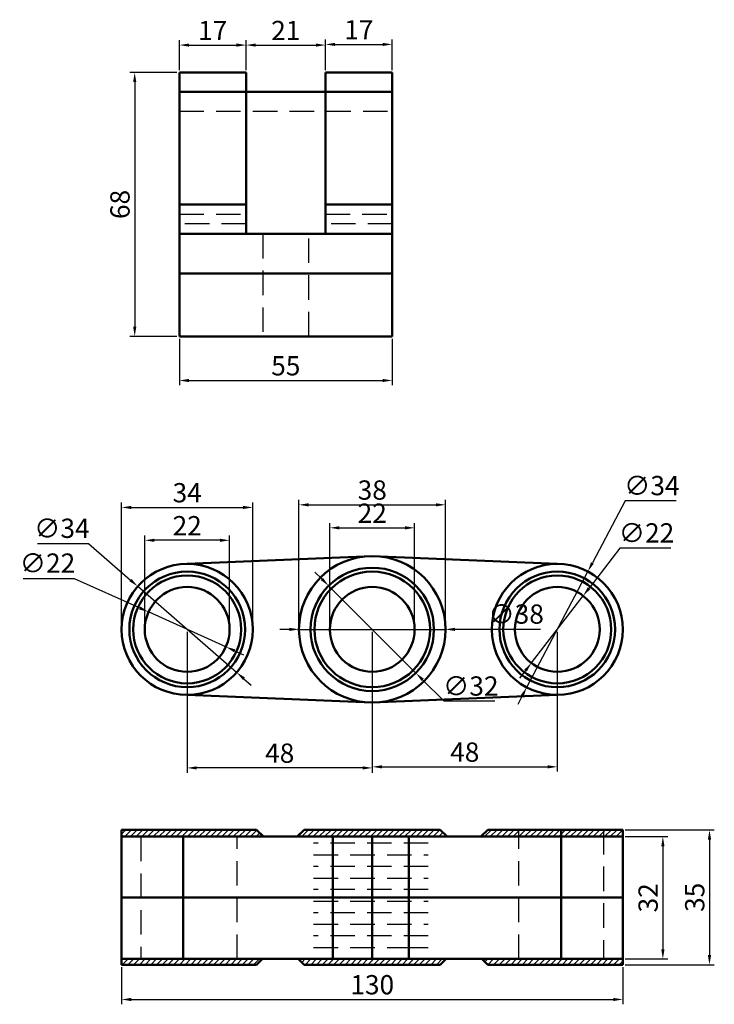
# Model space of a CAD drawing. Units: millimetres. Extents: x 1338 to 1892, y 1867 to 2306.
# Tile 3 of 3: x 1712 to 1892, y 2050 to 2306. Entities that reach past the tile are written whole.
import ezdxf

# ---------------------------------------------------------------- set-up
doc = ezdxf.new("R2010")
doc.units = ezdxf.units.MM
doc.linetypes.add('HIDDEN', pattern=[9.525, 6.35, -3.175])
for name, color, linetype, lineweight in [('M-DIMS', 2, 'Continuous', 25), ('M-HATC', 8, 'Continuous', 18), ('M-HIDN', 4, 'HIDDEN', 25), ('M-OUTL', 7, 'Continuous', 50)]:
    doc.layers.add(name, color=color, linetype=linetype, lineweight=lineweight)
doc.styles.get("Standard").update_dxf_attribs({"font": 'arial.ttf'})
doc.dimstyles.new('ISO-25', dxfattribs={"dimtxt": 5, "dimasz": 2.5, "dimexe": 1.25, "dimexo": 0.625, "dimtad": 1, "dimtoh": 1, "dimdec": 0, "dimtxsty": 'Standard', "dimcen": 2.5, "dimadec": 0, "dimazin": 0, "dimtfac": 1, "dimtdec": 0, "dimtmove": 0, "dimatfit": 3, "dimfxl": 1, "dimarcsym": 0})

# ---------------------------------------------------------------- blocks, each defined once
blk = doc.blocks.new('*D26')
at = {"layer": 'Defpoints', "color": 0, "transparency": 16777216}
for p in [(1771.04, 2299.06), (1753.74, 2291.96), (1771.04, 2291.96)]:
    blk.add_point(p, dxfattribs=at)
at = {"layer": 'M-DIMS', "color": 0, "lineweight": -2, "transparency": 16777216}
for p, q in [((1753.74, 2292.59), (1753.74, 2300.31)), ((1756.24, 2299.06), (1768.54, 2299.06)), ((1771.04, 2292.59), (1771.04, 2300.31))]:
    blk.add_line(p, q, dxfattribs=at)
at = {"layer": 'M-DIMS', "color": 0, "transparency": 16777216}
for points in [[(1756.24, 2299.48), (1756.24, 2298.65), (1753.74, 2299.06)], [(1768.54, 2299.48), (1768.54, 2298.65), (1771.04, 2299.06)]]:
    blk.add_solid(points, dxfattribs=at)
at = {"layer": 'M-DIMS', "color": 0, "transparency": 16777216, "insert": (1762.39, 2302.2), "char_height": 5, "attachment_point": 5}
blk.add_mtext('17', dxfattribs=at)
blk = doc.blocks.new('*D27')
at = {"layer": 'Defpoints', "color": 0, "transparency": 16777216}
for p in [(1791.64, 2299.06), (1771.04, 2291.96), (1791.64, 2291.96)]:
    blk.add_point(p, dxfattribs=at)
at = {"layer": 'M-DIMS', "color": 0, "lineweight": -2, "transparency": 16777216}
for p, q in [((1771.04, 2292.59), (1771.04, 2300.31)), ((1773.54, 2299.06), (1789.14, 2299.06)), ((1791.64, 2292.59), (1791.64, 2300.31))]:
    blk.add_line(p, q, dxfattribs=at)
at = {"layer": 'M-DIMS', "color": 0, "transparency": 16777216}
for points in [[(1773.54, 2299.48), (1773.54, 2298.65), (1771.04, 2299.06)], [(1789.14, 2299.48), (1789.14, 2298.65), (1791.64, 2299.06)]]:
    blk.add_solid(points, dxfattribs=at)
at = {"layer": 'M-DIMS', "color": 0, "transparency": 16777216, "insert": (1781.34, 2302.2), "char_height": 5, "attachment_point": 5}
blk.add_mtext('21', dxfattribs=at)
blk = doc.blocks.new('*D28')
at = {"layer": 'Defpoints', "color": 0, "transparency": 16777216}
for p in [(1808.94, 2299.23), (1791.64, 2291.96), (1808.94, 2291.96)]:
    blk.add_point(p, dxfattribs=at)
at = {"layer": 'M-DIMS', "color": 0, "lineweight": -2, "transparency": 16777216}
for p, q in [((1791.64, 2292.59), (1791.64, 2300.48)), ((1794.14, 2299.23), (1806.44, 2299.23)), ((1808.94, 2292.59), (1808.94, 2300.48))]:
    blk.add_line(p, q, dxfattribs=at)
at = {"layer": 'M-DIMS', "color": 0, "transparency": 16777216}
for points in [[(1794.14, 2299.65), (1794.14, 2298.82), (1791.64, 2299.23)], [(1806.44, 2299.65), (1806.44, 2298.82), (1808.94, 2299.23)]]:
    blk.add_solid(points, dxfattribs=at)
at = {"layer": 'M-DIMS', "color": 0, "transparency": 16777216, "insert": (1800.29, 2302.37), "char_height": 5, "attachment_point": 5}
blk.add_mtext('17', dxfattribs=at)
blk = doc.blocks.new('*D29')
at = {"layer": 'Defpoints', "color": 0, "transparency": 16777216}
for p in [(1753.74, 2291.96), (1742.15, 2223.49), (1753.74, 2223.49)]:
    blk.add_point(p, dxfattribs=at)
at = {"layer": 'M-DIMS', "color": 0, "lineweight": -2, "transparency": 16777216}
for p, q in [((1753.12, 2291.96), (1740.9, 2291.96)), ((1742.15, 2289.46), (1742.15, 2225.99)), ((1753.12, 2223.49), (1740.9, 2223.49))]:
    blk.add_line(p, q, dxfattribs=at)
at = {"layer": 'M-DIMS', "color": 0, "transparency": 16777216}
for points in [[(1741.74, 2289.46), (1742.57, 2289.46), (1742.15, 2291.96)], [(1741.74, 2225.99), (1742.57, 2225.99), (1742.15, 2223.49)]]:
    blk.add_solid(points, dxfattribs=at)
at = {"layer": 'M-DIMS', "color": 0, "transparency": 16777216, "insert": (1738.98, 2257.72), "char_height": 5, "attachment_point": 5, "rotation": 90}
blk.add_mtext('68', dxfattribs=at)
blk = doc.blocks.new('*D30')
at = {"layer": 'Defpoints', "color": 0, "transparency": 16777216}
for p in [(1753.74, 2223.49), (1808.94, 2223.49), (1808.94, 2212.04)]:
    blk.add_point(p, dxfattribs=at)
at = {"layer": 'M-DIMS', "color": 0, "lineweight": -2, "transparency": 16777216}
for p, q in [((1753.74, 2222.86), (1753.74, 2210.79)), ((1808.94, 2222.86), (1808.94, 2210.79)), ((1756.24, 2212.04), (1806.44, 2212.04))]:
    blk.add_line(p, q, dxfattribs=at)
at = {"layer": 'M-DIMS', "color": 0, "transparency": 16777216}
for points in [[(1756.24, 2212.46), (1756.24, 2211.63), (1753.74, 2212.04)], [(1806.44, 2212.46), (1806.44, 2211.63), (1808.94, 2212.04)]]:
    blk.add_solid(points, dxfattribs=at)
at = {"layer": 'M-DIMS', "color": 0, "transparency": 16777216, "insert": (1781.34, 2215.21), "char_height": 5, "attachment_point": 5}
blk.add_mtext('55', dxfattribs=at)
blk = doc.blocks.new('*D31')
at = {"layer": 'Defpoints', "color": 0, "transparency": 16777216}
for p in [(1772.76, 2179.1), (1738.76, 2147.47), (1772.76, 2147.47)]:
    blk.add_point(p, dxfattribs=at)
at = {"layer": 'M-DIMS', "color": 0, "lineweight": -2, "transparency": 16777216}
for p, q in [((1738.76, 2148.09), (1738.76, 2180.35)), ((1741.26, 2179.1), (1770.26, 2179.1)), ((1772.76, 2148.09), (1772.76, 2180.35))]:
    blk.add_line(p, q, dxfattribs=at)
at = {"layer": 'M-DIMS', "color": 0, "transparency": 16777216}
for points in [[(1741.26, 2179.52), (1741.26, 2178.69), (1738.76, 2179.1)], [(1770.26, 2179.52), (1770.26, 2178.69), (1772.76, 2179.1)]]:
    blk.add_solid(points, dxfattribs=at)
at = {"layer": 'M-DIMS', "color": 0, "transparency": 16777216, "insert": (1755.76, 2182.28), "char_height": 5, "attachment_point": 5}
blk.add_mtext('34', dxfattribs=at)
blk = doc.blocks.new('*D32')
at = {"layer": 'Defpoints', "color": 0, "transparency": 16777216}
for p in [(1822.76, 2179.79), (1784.76, 2147.47), (1822.76, 2147.47)]:
    blk.add_point(p, dxfattribs=at)
at = {"layer": 'M-DIMS', "color": 0, "lineweight": -2, "transparency": 16777216}
for p, q in [((1784.76, 2148.09), (1784.76, 2181.04)), ((1787.26, 2179.79), (1820.26, 2179.79)), ((1822.76, 2148.09), (1822.76, 2181.04))]:
    blk.add_line(p, q, dxfattribs=at)
at = {"layer": 'M-DIMS', "color": 0, "transparency": 16777216}
for points in [[(1787.26, 2180.2), (1787.26, 2179.37), (1784.76, 2179.79)], [(1820.26, 2180.2), (1820.26, 2179.37), (1822.76, 2179.79)]]:
    blk.add_solid(points, dxfattribs=at)
at = {"layer": 'M-DIMS', "color": 0, "transparency": 16777216, "insert": (1803.76, 2182.97), "char_height": 5, "attachment_point": 5}
blk.add_mtext('38', dxfattribs=at)
blk = doc.blocks.new('*D33')
at = {"layer": 'Defpoints', "color": 0, "transparency": 16777216}
for p in [(1744.76, 2170.58), (1744.76, 2147.47), (1766.76, 2147.47)]:
    blk.add_point(p, dxfattribs=at)
at = {"layer": 'M-DIMS', "color": 0, "lineweight": -2, "transparency": 16777216}
for p, q in [((1744.76, 2148.09), (1744.76, 2171.83)), ((1766.76, 2148.09), (1766.76, 2171.83)), ((1764.26, 2170.58), (1747.26, 2170.58))]:
    blk.add_line(p, q, dxfattribs=at)
at = {"layer": 'M-DIMS', "color": 0, "transparency": 16777216}
for points in [[(1747.26, 2171), (1747.26, 2170.17), (1744.76, 2170.58)], [(1764.26, 2171), (1764.26, 2170.17), (1766.76, 2170.58)]]:
    blk.add_solid(points, dxfattribs=at)
at = {"layer": 'M-DIMS', "color": 0, "transparency": 16777216, "insert": (1755.76, 2173.72), "char_height": 5, "attachment_point": 5}
blk.add_mtext('22', dxfattribs=at)
blk = doc.blocks.new('*D34')
at = {"layer": 'Defpoints', "color": 0, "transparency": 16777216}
for p in [(1814.76, 2173.82), (1792.76, 2147.47), (1814.76, 2147.47)]:
    blk.add_point(p, dxfattribs=at)
at = {"layer": 'M-DIMS', "color": 0, "lineweight": -2, "transparency": 16777216}
for p, q in [((1792.76, 2148.09), (1792.76, 2175.07)), ((1814.76, 2148.09), (1814.76, 2175.07)), ((1795.26, 2173.82), (1812.26, 2173.82))]:
    blk.add_line(p, q, dxfattribs=at)
at = {"layer": 'M-DIMS', "color": 0, "transparency": 16777216}
for points in [[(1795.26, 2174.24), (1795.26, 2173.4), (1792.76, 2173.82)], [(1812.26, 2174.24), (1812.26, 2173.4), (1814.76, 2173.82)]]:
    blk.add_solid(points, dxfattribs=at)
at = {"layer": 'M-DIMS', "color": 0, "transparency": 16777216, "insert": (1803.76, 2176.96), "char_height": 5, "attachment_point": 5}
blk.add_mtext('22', dxfattribs=at)
blk = doc.blocks.new('*D35')
at = {"layer": 'Defpoints', "color": 0, "transparency": 16777216}
for p in [(1742.94, 2158.63), (1768.59, 2136.31)]:
    blk.add_point(p, dxfattribs=at)
at = {"layer": 'M-DIMS', "color": 0, "lineweight": -2, "transparency": 16777216}
for p, q in [((1716.96, 2169.73), (1730.17, 2169.73)), ((1730.17, 2169.73), (1741.05, 2160.27)), ((1768.59, 2136.31), (1742.94, 2158.63)), ((1770.47, 2134.67), (1772.36, 2133.03))]:
    blk.add_line(p, q, dxfattribs=at)
at = {"layer": 'M-DIMS', "color": 0, "transparency": 16777216}
for points in [[(1741.32, 2160.58), (1740.78, 2159.95), (1742.94, 2158.63)], [(1770.75, 2134.99), (1770.2, 2134.36), (1768.59, 2136.31)]]:
    blk.add_solid(points, dxfattribs=at)
at = {"layer": 'M-DIMS', "color": 0, "transparency": 16777216, "insert": (1723.25, 2173.05), "char_height": 5, "attachment_point": 5}
blk.add_mtext('∅34', dxfattribs=at)
blk = doc.blocks.new('*D36')
at = {"layer": 'Defpoints', "color": 0, "transparency": 16777216}
for p in [(1745.73, 2151.99), (1765.79, 2142.95)]:
    blk.add_point(p, dxfattribs=at)
at = {"layer": 'M-DIMS', "color": 0, "lineweight": -2, "transparency": 16777216}
for p, q in [((1713.24, 2160.7), (1726.42, 2160.7)), ((1726.42, 2160.7), (1743.45, 2153.02)), ((1765.79, 2142.95), (1745.73, 2151.99)), ((1768.07, 2141.92), (1770.35, 2140.89))]:
    blk.add_line(p, q, dxfattribs=at)
at = {"layer": 'M-DIMS', "color": 0, "transparency": 16777216}
for points in [[(1743.63, 2153.4), (1743.28, 2152.64), (1745.73, 2151.99)], [(1768.24, 2142.3), (1767.9, 2141.54), (1765.79, 2142.95)]]:
    blk.add_solid(points, dxfattribs=at)
at = {"layer": 'M-DIMS', "color": 0, "transparency": 16777216, "insert": (1719.52, 2164.02), "char_height": 5, "attachment_point": 5}
blk.add_mtext('∅22', dxfattribs=at)
blk = doc.blocks.new('*D37')
at = {"layer": 'Defpoints', "color": 0, "transparency": 16777216}
for p in [(1858.48, 2156.18), (1845.05, 2138.76)]:
    blk.add_point(p, dxfattribs=at)
at = {"layer": 'M-DIMS', "color": 0, "lineweight": -2, "transparency": 16777216}
for p, q in [((1868, 2168.54), (1860, 2158.16)), ((1881.17, 2168.54), (1868, 2168.54)), ((1845.05, 2138.76), (1858.48, 2156.18)), ((1843.52, 2136.78), (1841.99, 2134.8))]:
    blk.add_line(p, q, dxfattribs=at)
at = {"layer": 'M-DIMS', "color": 0, "transparency": 16777216}
for points in [[(1859.67, 2158.42), (1860.33, 2157.91), (1858.48, 2156.18)], [(1843.19, 2137.03), (1843.85, 2136.52), (1845.05, 2138.76)]]:
    blk.add_solid(points, dxfattribs=at)
at = {"layer": 'M-DIMS', "color": 0, "transparency": 16777216, "insert": (1874.9, 2171.86), "char_height": 5, "attachment_point": 5}
blk.add_mtext('∅22', dxfattribs=at)
blk = doc.blocks.new('*D38')
at = {"layer": 'Defpoints', "color": 0, "transparency": 16777216}
for p in [(1859.7, 2162.5), (1843.82, 2132.44)]:
    blk.add_point(p, dxfattribs=at)
at = {"layer": 'M-DIMS', "color": 0, "lineweight": -2, "transparency": 16777216}
for p, q in [((1869.36, 2180.81), (1860.87, 2164.71)), ((1882.57, 2180.81), (1869.36, 2180.81)), ((1843.82, 2132.44), (1859.7, 2162.5)), ((1842.66, 2130.22), (1841.49, 2128.01))]:
    blk.add_line(p, q, dxfattribs=at)
at = {"layer": 'M-DIMS', "color": 0, "transparency": 16777216}
for points in [[(1860.5, 2164.91), (1861.23, 2164.52), (1859.7, 2162.5)], [(1842.29, 2130.42), (1843.03, 2130.03), (1843.82, 2132.44)]]:
    blk.add_solid(points, dxfattribs=at)
at = {"layer": 'M-DIMS', "color": 0, "transparency": 16777216, "insert": (1876.28, 2184.13), "char_height": 5, "attachment_point": 5}
blk.add_mtext('∅34', dxfattribs=at)
blk = doc.blocks.new('*D39')
at = {"layer": 'Defpoints', "color": 0, "transparency": 16777216}
for p in [(1803.76, 2147.47), (1851.76, 2147.47), (1851.76, 2111.81)]:
    blk.add_point(p, dxfattribs=at)
at = {"layer": 'M-DIMS', "color": 0, "lineweight": -2, "transparency": 16777216}
for p, q in [((1803.76, 2146.84), (1803.76, 2110.56)), ((1851.76, 2146.84), (1851.76, 2110.56)), ((1806.26, 2111.81), (1849.26, 2111.81))]:
    blk.add_line(p, q, dxfattribs=at)
at = {"layer": 'M-DIMS', "color": 0, "transparency": 16777216}
for points in [[(1806.26, 2112.22), (1806.26, 2111.39), (1803.76, 2111.81)], [(1849.26, 2112.22), (1849.26, 2111.39), (1851.76, 2111.81)]]:
    blk.add_solid(points, dxfattribs=at)
at = {"layer": 'M-DIMS', "color": 0, "transparency": 16777216, "insert": (1827.76, 2114.98), "char_height": 5, "attachment_point": 5}
blk.add_mtext('48', dxfattribs=at)
blk = doc.blocks.new('*D40')
at = {"layer": 'Defpoints', "color": 0, "transparency": 16777216}
for p in [(1755.76, 2147.47), (1803.76, 2147.47), (1755.76, 2111.53)]:
    blk.add_point(p, dxfattribs=at)
at = {"layer": 'M-DIMS', "color": 0, "lineweight": -2, "transparency": 16777216}
for p, q in [((1755.76, 2146.84), (1755.76, 2110.28)), ((1803.76, 2146.84), (1803.76, 2110.28)), ((1801.26, 2111.53), (1758.26, 2111.53))]:
    blk.add_line(p, q, dxfattribs=at)
at = {"layer": 'M-DIMS', "color": 0, "transparency": 16777216}
for points in [[(1758.26, 2111.95), (1758.26, 2111.12), (1755.76, 2111.53)], [(1801.26, 2111.95), (1801.26, 2111.12), (1803.76, 2111.53)]]:
    blk.add_solid(points, dxfattribs=at)
at = {"layer": 'M-DIMS', "color": 0, "transparency": 16777216, "insert": (1779.76, 2114.71), "char_height": 5, "attachment_point": 5}
blk.add_mtext('48', dxfattribs=at)
blk = doc.blocks.new('*D41')
at = {"layer": 'Defpoints', "color": 0, "transparency": 16777216}
for p in [(1868.76, 2095.45), (1868.76, 2060.45), (1891.24, 2060.45)]:
    blk.add_point(p, dxfattribs=at)
at = {"layer": 'M-DIMS', "color": 0, "lineweight": -2, "transparency": 16777216}
for p, q in [((1869.39, 2095.45), (1892.49, 2095.45)), ((1891.24, 2092.95), (1891.24, 2062.95)), ((1869.39, 2060.45), (1892.49, 2060.45))]:
    blk.add_line(p, q, dxfattribs=at)
at = {"layer": 'M-DIMS', "color": 0, "transparency": 16777216}
for points in [[(1890.82, 2092.95), (1891.65, 2092.95), (1891.24, 2095.45)], [(1890.82, 2062.95), (1891.65, 2062.95), (1891.24, 2060.45)]]:
    blk.add_solid(points, dxfattribs=at)
at = {"layer": 'M-DIMS', "color": 0, "transparency": 16777216, "insert": (1888.06, 2077.95), "char_height": 5, "attachment_point": 5, "rotation": 90}
blk.add_mtext('35', dxfattribs=at)
blk = doc.blocks.new('*D42')
at = {"layer": 'Defpoints', "color": 0, "transparency": 16777216}
for p in [(1868.76, 2093.7), (1868.76, 2061.96), (1879.15, 2061.96)]:
    blk.add_point(p, dxfattribs=at)
at = {"layer": 'M-DIMS', "color": 0, "lineweight": -2, "transparency": 16777216}
for p, q in [((1869.39, 2093.7), (1880.4, 2093.7)), ((1879.15, 2091.2), (1879.15, 2064.46)), ((1869.39, 2061.96), (1880.4, 2061.96))]:
    blk.add_line(p, q, dxfattribs=at)
at = {"layer": 'M-DIMS', "color": 0, "transparency": 16777216}
for points in [[(1878.74, 2091.2), (1879.57, 2091.2), (1879.15, 2093.7)], [(1878.74, 2064.46), (1879.57, 2064.46), (1879.15, 2061.96)]]:
    blk.add_solid(points, dxfattribs=at)
at = {"layer": 'M-DIMS', "color": 0, "transparency": 16777216, "insert": (1875.97, 2077.83), "char_height": 5, "attachment_point": 5, "rotation": 90}
blk.add_mtext('32', dxfattribs=at)
blk = doc.blocks.new('*D57')
at = {"layer": 'Defpoints', "color": 0, "transparency": 16777216}
for p in [(1738.76, 2060.45), (1868.76, 2060.45), (1868.76, 2051.45)]:
    blk.add_point(p, dxfattribs=at)
at = {"layer": 'M-DIMS', "color": 0, "lineweight": -2, "transparency": 16777216}
for p, q in [((1738.76, 2059.82), (1738.76, 2050.2)), ((1868.76, 2059.82), (1868.76, 2050.2)), ((1741.26, 2051.45), (1866.26, 2051.45))]:
    blk.add_line(p, q, dxfattribs=at)
at = {"layer": 'M-DIMS', "color": 0, "transparency": 16777216}
for points in [[(1741.26, 2051.87), (1741.26, 2051.03), (1738.76, 2051.45)], [(1866.26, 2051.87), (1866.26, 2051.03), (1868.76, 2051.45)]]:
    blk.add_solid(points, dxfattribs=at)
at = {"layer": 'M-DIMS', "color": 0, "transparency": 16777216, "insert": (1803.76, 2054.63), "char_height": 5, "attachment_point": 5}
blk.add_mtext('130', dxfattribs=at)
blk = doc.blocks.new('*D74')
at = {"layer": 'Defpoints', "color": 0, "transparency": 16777216}
for p in [(1792.45, 2158.78), (1815.08, 2136.15)]:
    blk.add_point(p, dxfattribs=at)
at = {"layer": 'M-DIMS', "color": 0, "lineweight": -2, "transparency": 16777216}
for p, q in [((1790.68, 2160.55), (1788.91, 2162.32)), ((1792.45, 2158.78), (1815.08, 2136.15)), ((1822.42, 2128.81), (1816.84, 2134.39)), ((1835.59, 2128.81), (1822.42, 2128.81))]:
    blk.add_line(p, q, dxfattribs=at)
at = {"layer": 'M-DIMS', "color": 0, "transparency": 16777216}
for points in [[(1790.98, 2160.85), (1790.39, 2160.26), (1792.45, 2158.78)], [(1817.14, 2134.68), (1816.55, 2134.09), (1815.08, 2136.15)]]:
    blk.add_solid(points, dxfattribs=at)
at = {"layer": 'M-DIMS', "color": 0, "transparency": 16777216, "insert": (1829.32, 2132.13), "char_height": 5, "attachment_point": 5}
blk.add_mtext('∅32', dxfattribs=at)
blk = doc.blocks.new('*D75')
at = {"layer": 'Defpoints', "color": 0, "transparency": 16777216}
for p in [(1784.76, 2147.47), (1822.76, 2147.47)]:
    blk.add_point(p, dxfattribs=at)
at = {"layer": 'M-DIMS', "color": 0, "lineweight": -2, "transparency": 16777216}
for p, q in [((1782.26, 2147.47), (1779.76, 2147.47)), ((1784.76, 2147.47), (1822.76, 2147.47)), ((1834.16, 2147.47), (1825.26, 2147.47)), ((1847.4, 2147.47), (1834.16, 2147.47))]:
    blk.add_line(p, q, dxfattribs=at)
at = {"layer": 'M-DIMS', "color": 0, "transparency": 16777216}
for points in [[(1782.26, 2147.89), (1782.26, 2147.05), (1784.76, 2147.47)], [(1825.26, 2147.89), (1825.26, 2147.05), (1822.76, 2147.47)]]:
    blk.add_solid(points, dxfattribs=at)
at = {"layer": 'M-DIMS', "color": 0, "transparency": 16777216, "insert": (1841.09, 2150.79), "char_height": 5, "attachment_point": 5}
blk.add_mtext('∅38', dxfattribs=at)

msp = doc.modelspace()

# ---------------------------------------------------------------- hatches: boundary and pattern name
at = {"layer": 'M-HATC'}
h = msp.add_hatch(dxfattribs=at)
h.set_pattern_fill('ANSI31', color=256, scale=0.33)
h.paths.add_polyline_path([(1773.762, 2095.449), (1738.762, 2095.449), (1738.762, 2093.697), (1775.572, 2093.697)])
h.paths.add_polyline_path([(1821.396, 2095.449), (1786.128, 2095.449), (1784.311, 2093.697), (1823.213, 2093.697)])
h.paths.add_polyline_path([(1841.762, 2095.449), (1833.762, 2095.449), (1831.951, 2093.697), (1841.762, 2093.697)])
h.paths.add_polyline_path([(1852.762, 2095.449), (1841.762, 2095.449), (1841.762, 2093.697), (1852.762, 2093.697)])
h.paths.add_polyline_path([(1863.762, 2095.449), (1852.762, 2095.449), (1852.762, 2093.697), (1863.762, 2093.697)])
h.paths.add_polyline_path([(1868.762, 2095.449), (1863.762, 2095.449), (1863.762, 2093.697), (1868.762, 2093.697)])
h.paths.add_polyline_path([(1768.762, 2061.964), (1738.762, 2061.964), (1738.762, 2060.449), (1768.762, 2060.449)])
h.paths.add_polyline_path([(1775.327, 2061.964), (1768.762, 2061.964), (1768.762, 2060.449), (1773.762, 2060.449)])
h.paths.add_polyline_path([(1822.961, 2061.964), (1784.562, 2061.964), (1786.128, 2060.449), (1821.396, 2060.449)])
h.paths.add_polyline_path([(1841.762, 2061.964), (1832.197, 2061.964), (1833.762, 2060.449), (1841.762, 2060.449)])
h.paths.add_polyline_path([(1852.762, 2061.964), (1841.762, 2061.964), (1841.762, 2060.449), (1852.762, 2060.449)])
h.paths.add_polyline_path([(1863.762, 2061.964), (1852.762, 2061.964), (1852.762, 2060.449), (1863.762, 2060.449)])
h.paths.add_polyline_path([(1868.762, 2061.964), (1863.762, 2061.964), (1863.762, 2060.449), (1868.762, 2060.449)])

# ---------------------------------------------------------------- linework, layer by layer
at = {"layer": 'M-HIDN'}
for p, q in [((1753.745, 2286.961), (1753.745, 2281.961)), ((1753.745, 2281.961), (1808.945, 2281.961)), ((1753.745, 2257.725), (1753.745, 2255.225)), ((1753.745, 2255.225), (1771.045, 2255.225)), ((1791.645, 2255.225), (1808.945, 2255.225)), ((1771.045, 2252.725), (1753.745, 2252.725)), ((1808.945, 2252.725), (1791.645, 2252.725)), ((1781.345, 2250.068), (1775.345, 2250.068)), ((1775.345, 2250.068), (1775.345, 2223.488)), ((1787.345, 2223.488), (1787.345, 2250.068)), ((1738.762, 2095.449), (1743.762, 2095.449)), ((1841.762, 2061.964), (1841.762, 2095.449)), ((1868.762, 2095.449), (1863.762, 2095.449)), ((1863.762, 2095.449), (1863.762, 2061.964)), ((1743.762, 2093.697), (1743.762, 2061.964)), ((1768.762, 2061.964), (1768.762, 2093.697)), ((1818.294, 2091.964), (1788.542, 2091.964)), ((1788.542, 2088.964), (1818.294, 2088.964)), ((1818.294, 2085.964), (1788.542, 2085.964)), ((1788.542, 2082.964), (1818.294, 2082.964)), ((1818.294, 2079.964), (1788.542, 2079.964)), ((1788.542, 2076.964), (1818.294, 2076.964)), ((1818.294, 2073.964), (1788.542, 2073.964)), ((1788.542, 2070.964), (1818.294, 2070.964)), ((1818.294, 2067.964), (1788.542, 2067.964)), ((1788.542, 2064.964), (1813.294, 2064.964)), ((1813.294, 2064.964), (1818.294, 2064.964)), ((1793.542, 2061.964), (1788.542, 2061.964))]:
    msp.add_line(p, q, dxfattribs=at)
at = {"layer": 'M-OUTL'}
for p, q in [((1753.745, 2291.961), (1771.045, 2291.961)), ((1753.745, 2291.961), (1753.745, 2223.488)), ((1753.745, 2291.961), (1753.745, 2286.961)), ((1771.045, 2291.961), (1771.045, 2250.068)), ((1791.645, 2250.068), (1791.645, 2291.961)), ((1791.645, 2291.961), (1808.945, 2291.961)), ((1808.945, 2291.961), (1808.945, 2228.961)), ((1753.745, 2286.961), (1808.945, 2286.961)), ((1753.745, 2257.725), (1771.045, 2257.725)), ((1791.645, 2257.725), (1808.945, 2257.725)), ((1771.045, 2250.068), (1753.745, 2250.068)), ((1771.045, 2250.068), (1791.645, 2250.068)), ((1791.645, 2250.068), (1808.945, 2250.068)), ((1771.045, 2239.825), (1753.745, 2239.825)), ((1771.045, 2239.825), (1791.645, 2239.825)), ((1791.645, 2239.825), (1808.945, 2239.825)), ((1808.945, 2228.961), (1808.945, 2223.488)), ((1753.745, 2223.488), (1808.945, 2223.488)), ((1803.762, 2166.469), (1755.762, 2164.469)), ((1803.762, 2166.469), (1851.762, 2164.469)), ((1755.762, 2130.469), (1803.762, 2128.469)), ((1803.762, 2128.469), (1851.762, 2130.469)), ((1738.762, 2095.449), (1773.762, 2095.449)), ((1738.762, 2095.449), (1738.762, 2060.449)), ((1743.762, 2095.449), (1754.762, 2095.449)), ((1773.762, 2095.449), (1775.327, 2093.935)), ((1773.762, 2095.449), (1775.572, 2093.697)), ((1786.128, 2095.449), (1784.311, 2093.697)), ((1786.128, 2095.449), (1784.562, 2093.935)), ((1786.128, 2095.449), (1821.396, 2095.449)), ((1821.396, 2095.449), (1823.213, 2093.697)), ((1833.762, 2095.449), (1831.951, 2093.697)), ((1833.762, 2095.449), (1868.762, 2095.449)), ((1863.762, 2095.449), (1852.762, 2095.449)), ((1852.762, 2095.449), (1852.762, 2061.964)), ((1868.762, 2095.449), (1868.762, 2060.449)), ((1738.762, 2093.697), (1868.762, 2093.697)), ((1754.762, 2093.697), (1754.762, 2061.964)), ((1793.542, 2093.697), (1793.542, 2061.964)), ((1803.762, 2093.697), (1803.762, 2061.964)), ((1813.294, 2093.697), (1813.294, 2061.964)), ((1738.762, 2077.949), (1868.762, 2077.949)), ((1738.762, 2061.964), (1868.762, 2061.964)), ((1773.762, 2060.449), (1775.327, 2061.964)), ((1786.128, 2060.449), (1784.562, 2061.964)), ((1821.396, 2060.449), (1822.961, 2061.964)), ((1833.762, 2060.449), (1832.197, 2061.964)), ((1738.762, 2060.449), (1773.762, 2060.449)), ((1768.762, 2060.449), (1773.762, 2060.449)), ((1786.128, 2060.449), (1821.396, 2060.449)), ((1833.762, 2060.449), (1868.762, 2060.449))]:
    msp.add_line(p, q, dxfattribs=at)
for centre, radius in [((1803.762, 2147.469), 19), ((1755.762, 2147.469), 17), ((1851.762, 2147.469), 17), ((1755.762, 2147.469), 15), ((1755.762, 2147.469), 14), ((1803.762, 2147.469), 16), ((1803.762, 2147.469), 15), ((1851.762, 2147.469), 15), ((1851.762, 2147.469), 14), ((1755.762, 2147.469), 11), ((1803.762, 2147.469), 11), ((1851.762, 2147.469), 11)]:
    msp.add_circle(centre, radius, dxfattribs=at)

# ---------------------------------------------------------------- dimensions: what is measured, and where the dimension line sits
at = {"layer": 'M-DIMS'}
for base, p1, p2, override, picture, middle in [((1771.045, 2299.065), (1753.745, 2291.961), (1771.045, 2291.961), {"dimclrd": 0, "dimclre": 0, "dimclrt": 0}, '*D26', (1762.395, 2302.2)), ((1791.645, 2299.065), (1771.045, 2291.961), (1791.645, 2291.961), {"dimclrd": 0, "dimclre": 0, "dimclrt": 0}, '*D27', (1781.345, 2302.2)), ((1808.945, 2299.234), (1791.645, 2291.961), (1808.945, 2291.961), {"dimclrd": 0, "dimclre": 0, "dimclrt": 0}, '*D28', (1800.295, 2302.369)), ((1808.945, 2212.043), (1753.745, 2223.488), (1808.945, 2223.488), {"dimclrd": 0, "dimclre": 0, "dimclrt": 0}, '*D30', (1781.345, 2215.211)), ((1772.762, 2179.105), (1738.762, 2147.469), (1772.762, 2147.469), {"dimclrd": 0, "dimclre": 0, "dimclrt": 0}, '*D31', (1755.762, 2182.284)), ((1822.762, 2179.786), (1784.762, 2147.469), (1822.762, 2147.469), {"dimclrd": 0, "dimclre": 0, "dimclrt": 0}, '*D32', (1803.762, 2182.966)), ((1814.762, 2173.821), (1792.762, 2147.469), (1814.762, 2147.469), {"dimclrd": 0, "dimclre": 0, "dimclrt": 0}, '*D34', (1803.762, 2176.956)), ((1744.762, 2170.583), (1766.762, 2147.469), (1744.762, 2147.469), {"dimclrd": 0, "dimclre": 0, "dimclrt": 0}, '*D33', (1755.762, 2173.718)), ((1755.762, 2111.532), (1803.762, 2147.469), (1755.762, 2147.469), {"dimclrd": 0, "dimclre": 0, "dimclrt": 0}, '*D40', (1779.762, 2114.71)), ((1851.762, 2111.805), (1803.762, 2147.469), (1851.762, 2147.469), {"dimclrd": 0, "dimclre": 0, "dimclrt": 0}, '*D39', (1827.762, 2114.983)), ((1868.762, 2051.449), (1738.762, 2060.449), (1868.762, 2060.449), {"dimdec": 0, "dimlfac": 1, "dimrnd": 0, "dimzin": 0, "dimdsep": 46, "dimlunit": 2}, '*D57', (1803.762, 2054.629))]:
    dim = msp.add_linear_dim(base=base, p1=p1, p2=p2, dimstyle='ISO-25', override=override, dxfattribs=at)
    dim.commit()
    dim.dimension.update_dxf_attribs({"geometry": picture, "text_midpoint": middle})
for base, p1, p2, picture, middle in [((1742.154, 2223.488), (1753.745, 2291.961), (1753.745, 2223.488), '*D29', (1738.976, 2257.725)), ((1891.236, 2060.449), (1868.762, 2095.449), (1868.762, 2060.449), '*D41', (1888.057, 2077.949)), ((1879.152, 2061.964), (1868.762, 2093.697), (1868.762, 2061.964), '*D42', (1875.973, 2077.831))]:
    dim = msp.add_linear_dim(base=base, p1=p1, p2=p2, angle=90, dimstyle='ISO-25', override={"dimclrd": 0, "dimclre": 0, "dimclrt": 0}, dxfattribs=at)
    dim.commit()
    dim.dimension.update_dxf_attribs({"geometry": picture, "text_midpoint": middle})
for p1, p2, override, picture, middle in [((1843.825, 2132.435), (1859.699, 2162.502), {"dimclrd": 0, "dimclre": 0, "dimclrt": 0}, '*D38', (1876.279, 2180.809)), ((1768.588, 2136.312), (1742.935, 2158.626), {"dimclrd": 0, "dimclre": 0, "dimclrt": 0}, '*D35', (1723.253, 2169.731)), ((1845.047, 2138.756), (1858.476, 2156.182), {"dimclrd": 0, "dimclre": 0, "dimclrt": 0}, '*D37', (1874.899, 2168.538)), ((1765.79, 2142.948), (1745.734, 2151.989), {"dimclrd": 0, "dimclre": 0, "dimclrt": 0}, '*D36', (1719.516, 2160.698)), ((1792.448, 2158.783), (1815.075, 2136.155), {"dimdec": 0, "dimlfac": 1, "dimrnd": 0, "dimzin": 0, "dimdsep": 46, "dimlunit": 2}, '*D74', (1829.319, 2128.811)), ((1784.762, 2147.469), (1822.762, 2147.469), {"dimdec": 0, "dimlfac": 1, "dimrnd": 0, "dimzin": 0, "dimdsep": 46, "dimlunit": 2}, '*D75', (1834.162, 2147.469))]:
    dim = msp.add_diameter_dim_2p(p1=p1, p2=p2, dimstyle='ISO-25', override=override, dxfattribs=at)
    dim.commit()
    dim.dimension.update_dxf_attribs({"geometry": picture, "text_midpoint": middle, "dimtype": 163})

doc.saveas('drawing.dxf')
